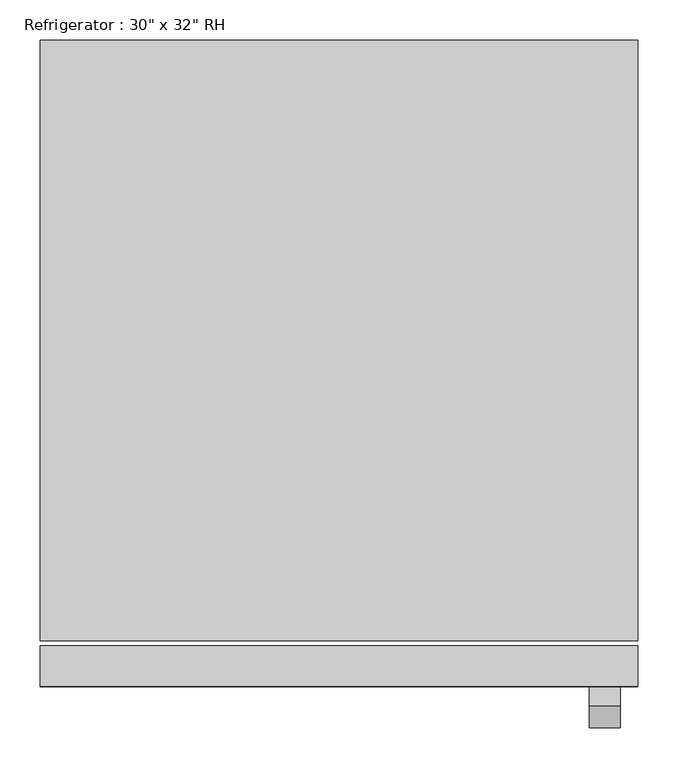
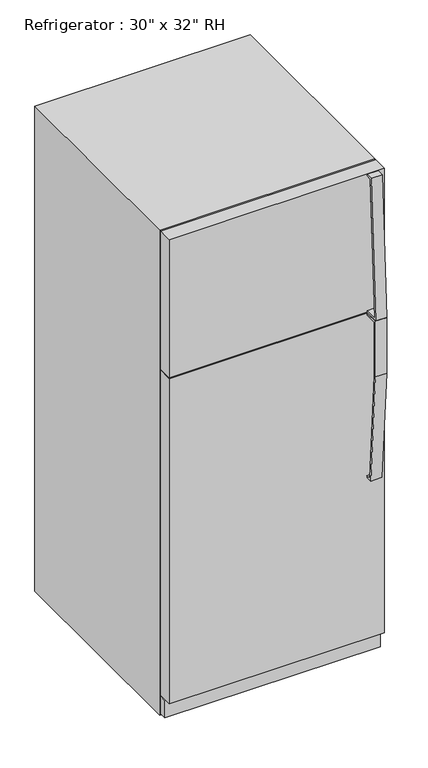
"""IFC4 building model written with IfcOpenShell, lengths in millimetres: proxy geometry."""

from ifc_helpers import new_model, si_unit, frame, origin, origin_with_axes, place, context, project, spatial, polyline, outline, extrude, source, transform, mapped, element, save


def proxy_a13a33b2(model_context):
    return source(origin(), model_context, "Body", "SweptSolid", [
        extrude(outline(polyline([(-417.9010285, 1262.0625), (-462.3510285, 1262.0625), (-462.3510285, 1065.4342469), (-434.8723987, 672.4715334), (-417.9010285, 672.4715334), (-417.9010285, 666.1370017), (-440.7949512, 666.1370017), (-468.7010285, 1065.2125), (-468.7010285, 1268.4125), (-417.9010285, 1268.4125), (-417.9010285, 1262.0625)])), frame((312.7375, 0.0, 0.0), z_axis=(1.0, 0.0, 0.0), x_axis=(0.0, 1.0, 0.0)), (0.0, 0.0, 1.0), 38.4332978),
        extrude(outline(polyline([(-442.739413, 1778.0), (-418.6780855, 1778.0), (-418.6780855, 1771.65), (-437.5263449, 1771.65), (-463.4007207, 1277.9375), (-418.6780855, 1277.9375), (-418.6780855, 1271.5875), (-469.2793675, 1271.5875), (-442.739413, 1778.0)])), frame((312.7375, 0.0, 0.0), z_axis=(1.0, 0.0, 0.0), x_axis=(0.0, 1.0, 0.0)), (0.0, 0.0, 1.0), 38.4332978),
        extrude(outline(polyline([(373.0625, -367.1010285), (373.0625, -392.5010285), (-373.0625, -392.5010285), (-373.0625, -367.1010285), (373.0625, -367.1010285)])), frame((0.0, 0.0, 9.3816357), z_axis=(0.0, 0.0, 1.0), x_axis=(1.0, 0.0, 0.0)), (0.0, 0.0, 1.0), 63.5),
        extrude(outline(polyline([(373.0625, -367.1010285), (373.0625, -417.9010285), (-373.0625, -417.9010285), (-373.0625, -367.1010285), (373.0625, -367.1010285)])), frame((0.0, 0.0, 76.2), z_axis=(0.0, 0.0, 1.0), x_axis=(1.0, 0.0, 0.0)), (0.0, 0.0, 1.0), 1192.2125),
        extrude(outline(polyline([(373.0625, -367.1010285), (373.0625, -417.9010285), (-373.0625, -417.9010285), (-373.0625, -367.1010285), (373.0625, -367.1010285)])), frame((0.0, 0.0, 1271.5875), z_axis=(0.0, 0.0, 1.0), x_axis=(1.0, 0.0, 0.0)), (0.0, 0.0, 1.0), 506.4125),
        extrude(outline(polyline([(373.0625, 388.5489715), (373.0625, -360.7510285), (-373.0625, -360.7510285), (-373.0625, 388.5489715), (373.0625, 388.5489715)])), origin_with_axes(), (0.0, 0.0, 1.0), 1778.0),
    ])


if __name__ == "__main__":
    model = new_model("IFC4")
    model_context = context("Model", 3, world=origin())
    ifc_project = project(units=[si_unit("LENGTHUNIT", "METRE", prefix="MILLI")], contexts=[model_context])
    site = spatial("IfcSite", under=ifc_project)
    building = spatial("IfcBuilding", under=site)
    placement = place(None, origin())
    proxy_shape = proxy_a13a33b2(model_context)
    element("IfcBuildingElementProxy", 1, Name="Refrigerator : 30\" x 32\" RH", ObjectType="Refrigerator : 30\" x 32\" RH", at=placement, inside=building, context=model_context, shape_type="MappedRepresentation", body=[
        mapped(proxy_shape, transform((0.0, 0.0, 0.0), x_axis=(1.0, 0.0, 0.0), y_axis=(0.0, 1.0, 0.0), z_axis=(0.0, 0.0, 1.0))),
    ])
    save(model, "model.ifc")

# Revit data of these elements
# Type "Refrigerator : 30\" x 32\" RH"
#   Label = "REF."
#   Assembly Code = "E1090400"
#   Depth = 2' - 7 3/4"
#   Handle = 2' - 3"
#   Height = 5' - 10"
#   Rear Clearance = 0' - 2"
#   Top Door Height = 1' - 8"
#   Width = 2' - 5 3/8"
#   Material = Steel, Chrome Plated
#   Default Elevation = 0
# Element 1 (IfcBuildingElementProxy, "Refrigerator : 30\" x 32\" RH")
#   Materials on its faces: "Steel, Chrome Plated"
# Materials
#   "Steel, Chrome Plated": class "Metal", colour RGB 17 17 17, transparency 0, Description = "Chromiuim plated steel", Cost = 0
